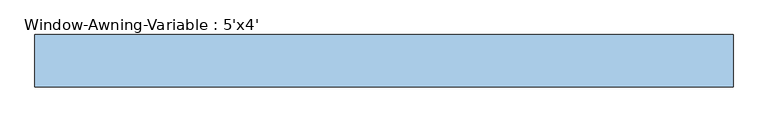
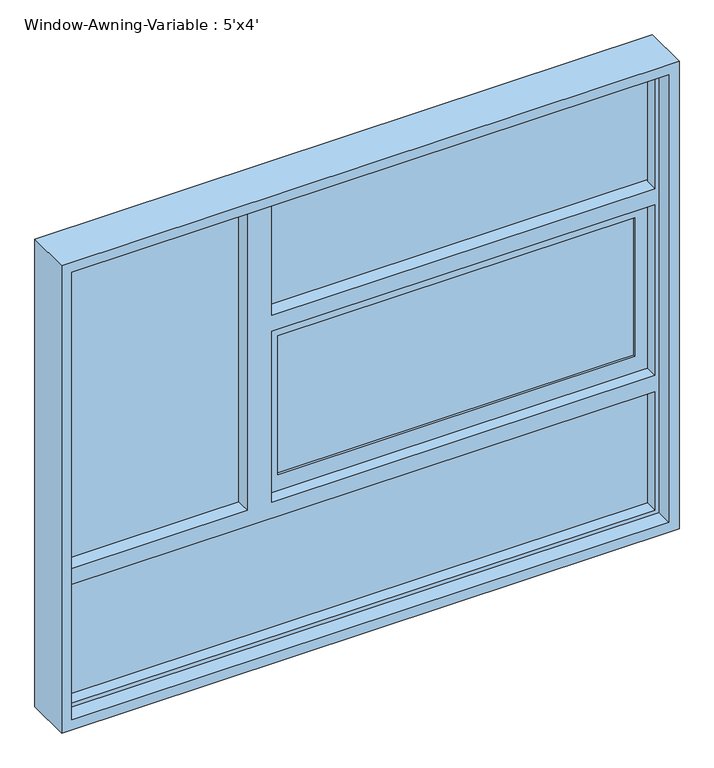
"""IFC4 building model written with IfcOpenShell, lengths in millimetres: window geometry, Window-Awning-Variable : 5'x4'."""

from ifc_helpers import new_model, si_unit, frame, origin, place, context, project, spatial, polyline, outline, extrude, faceted_brep, source, transform, mapped, element, save


def window_awning_variable_5_x4_55050b8f(model_context):
    return source(origin(), model_context, "Body", "SolidModel", [
        extrude(outline(polyline([(694.7296875, 41.275), (694.7296875, 34.925), (-186.7296875, 34.925), (-186.7296875, 41.275), (694.7296875, 41.275)])), frame((0.0, 0.0, 1342.9654688), z_axis=(0.0, 0.0, 1.0), x_axis=(1.0, 0.0, 0.0)), (0.0, 0.0, 1.0), 362.0690625),
        extrude(outline(polyline([(694.7296875, 28.575), (694.7296875, 22.225), (-186.7296875, 22.225), (-186.7296875, 28.575), (694.7296875, 28.575)])), frame((0.0, 0.0, 1342.9654688), z_axis=(0.0, 0.0, 1.0), x_axis=(1.0, 0.0, 0.0)), (0.0, 0.0, 1.0), 362.0690625),
        extrude(outline(polyline([(-279.4, 41.275), (-279.4, 34.925), (-736.6, 34.925), (-736.6, 41.275), (-279.4, 41.275)])), frame((0.0, 0.0, 1301.0951563), z_axis=(0.0, 0.0, 1.0), x_axis=(1.0, 0.0, 0.0)), (0.0, 0.0, 1.0), 807.1048438),
        extrude(outline(polyline([(-279.4, 28.575), (-279.4, 22.225), (-736.6, 22.225), (-736.6, 28.575), (-279.4, 28.575)])), frame((0.0, 0.0, 1301.0951563), z_axis=(0.0, 0.0, 1.0), x_axis=(1.0, 0.0, 0.0)), (0.0, 0.0, 1.0), 807.1048438),
        extrude(outline(polyline([(736.6, 28.575), (736.6, 22.225), (-228.6, 22.225), (-228.6, 28.575), (736.6, 28.575)])), frame((0.0, 0.0, 1788.7751563), z_axis=(0.0, 0.0, 1.0), x_axis=(1.0, 0.0, 0.0)), (0.0, 0.0, 1.0), 319.4248438),
        extrude(outline(polyline([(736.6, 41.275), (736.6, 34.925), (-228.6, 34.925), (-228.6, 41.275), (736.6, 41.275)])), frame((0.0, 0.0, 1788.7751563), z_axis=(0.0, 0.0, 1.0), x_axis=(1.0, 0.0, 0.0)), (0.0, 0.0, 1.0), 319.4248438),
        extrude(outline(polyline([(736.6, 41.275), (736.6, 34.925), (-736.6, 34.925), (-736.6, 41.275), (736.6, 41.275)])), frame((0.0, 0.0, 939.8), z_axis=(0.0, 0.0, 1.0), x_axis=(1.0, 0.0, 0.0)), (0.0, 0.0, 1.0), 319.4248438),
        extrude(outline(polyline([(736.6, 28.575), (736.6, 22.225), (-736.6, 22.225), (-736.6, 28.575), (736.6, 28.575)])), frame((0.0, 0.0, 939.8), z_axis=(0.0, 0.0, 1.0), x_axis=(1.0, 0.0, 0.0)), (0.0, 0.0, 1.0), 319.4248438),
        faceted_brep([(-736.6, 15.875, 2108.2), (-736.6, 57.15, 2108.2), (736.6, 57.15, 2108.2), (736.6, 15.875, 2108.2), (-228.6, 15.875, 2108.2), (-228.6, 53.975, 2108.2), (-279.4, 53.975, 2108.2), (-279.4, 15.875, 2108.2), (-726.4796875, -15.08125, 2098.0796875), (-726.4796875, 15.875, 2098.0796875), (-279.4, 15.875, 2098.0796875), (-279.4, -15.08125, 2098.0796875), (726.4796875, 15.875, 2098.0796875), (726.4796875, -15.08125, 2098.0796875), (-218.4796875, -15.08125, 2098.0796875), (-218.4796875, 15.875, 2098.0796875), (-736.6, -57.15, 2108.2), (-736.6, -15.08125, 2108.2), (736.6, -15.08125, 2108.2), (736.6, -57.15, 2108.2), (-762.0, 57.15, 2133.6), (-762.0, -57.15, 2133.6), (762.0, -57.15, 2133.6), (762.0, 57.15, 2133.6), (736.6, 57.15, 939.8), (736.6, 15.875, 939.8), (736.6, 15.875, 1259.2248438), (736.6, 53.975, 1259.2248438), (736.6, 53.975, 1301.0951563), (736.6, 15.875, 1301.0951563), (736.6, 15.875, 1746.9048438), (736.6, 53.975, 1746.9048438), (736.6, 53.975, 1788.7751563), (736.6, 15.875, 1788.7751563), (726.4796875, 15.875, 1788.7751563), (726.4796875, -15.08125, 1788.7751563), (726.4796875, 15.875, 949.9203125), (726.4796875, -15.08125, 949.9203125), (726.4796875, -15.08125, 1259.2248438), (726.4796875, 15.875, 1259.2248438), (726.4796875, 15.875, 1301.0951563), (726.4796875, -15.08125, 1301.0951563), (726.4796875, -15.08125, 1746.9048438), (726.4796875, 15.875, 1746.9048438), (736.6, -15.08125, 939.8), (736.6, -57.15, 939.8), (762.0, -57.15, 914.4), (762.0, 57.15, 914.4), (-736.6, 57.15, 939.8), (-736.6, 15.875, 939.8), (-726.4796875, 15.875, 949.9203125), (-726.4796875, -15.08125, 949.9203125), (-736.6, -15.08125, 939.8), (-736.6, -57.15, 939.8), (-762.0, -57.15, 914.4), (-762.0, 57.15, 914.4), (-736.6, 15.875, 1301.0951563), (-736.6, 53.975, 1301.0951563), (-736.6, 53.975, 1259.2248438), (-736.6, 15.875, 1259.2248438), (-218.4796875, 15.875, 1788.7751563), (-228.6, 15.875, 1788.7751563), (-726.4796875, 15.875, 1259.2248438), (-726.4796875, 15.875, 1301.0951563), (-218.4796875, 15.875, 1301.0951563), (-228.6, 15.875, 1301.0951563), (-228.6, 15.875, 1746.9048438), (-218.4796875, 15.875, 1746.9048438), (-726.4796875, -15.08125, 1301.0951563), (-726.4796875, -15.08125, 1259.2248438), (-218.4796875, -15.08125, 1788.7751563), (-279.4, -15.08125, 1301.0951563), (-218.4796875, -15.08125, 1301.0951563), (-218.4796875, -15.08125, 1746.9048438), (-279.4, 53.975, 1301.0951563), (-228.6, 53.975, 1788.7751563), (-228.6, 53.975, 1746.9048438), (-228.6, 53.975, 1301.0951563)], [[[0, 1, 2, 3, 4, 5, 6, 7]], [[8, 9, 10, 11]], [[12, 13, 14, 15]], [[16, 17, 18, 19]], [[20, 21, 22, 23]], [[3, 2, 24, 25, 26, 27, 28, 29, 30, 31, 32, 33]], [[13, 12, 34, 35]], [[36, 37, 38, 39]], [[40, 41, 42, 43]], [[19, 18, 44, 45]], [[23, 22, 46, 47]], [[25, 24, 48, 49]], [[37, 36, 50, 51]], [[45, 44, 52, 53]], [[47, 46, 54, 55]], [[1, 0, 56, 57, 58, 59, 49, 48]], [[12, 15, 60, 61, 4, 3, 33, 34]], [[25, 49, 59, 62, 50, 36, 39, 26]], [[56, 0, 7, 10, 9, 63]], [[29, 40, 43, 30]], [[64, 65, 66, 67]], [[9, 8, 68, 63]], [[51, 50, 62, 69]], [[52, 44, 18, 17], [14, 13, 35, 70], [37, 51, 69, 38], [68, 8, 11, 71], [72, 73, 42, 41]], [[17, 16, 53, 52]], [[22, 21, 54, 46], [16, 19, 45, 53]], [[21, 20, 55, 54]], [[20, 23, 47, 55], [2, 1, 48, 24]], [[58, 27, 26, 39, 38, 69, 62, 59]], [[27, 58, 57, 74, 6, 5, 75, 32, 31, 76, 77, 28]], [[29, 28, 77, 65, 64, 72, 41, 40]], [[57, 56, 63, 68, 71, 74]], [[6, 74, 71, 11, 10, 7]], [[15, 14, 70, 60]], [[72, 64, 67, 73]], [[5, 4, 61, 75]], [[65, 77, 76, 66]], [[76, 31, 30, 43, 42, 73, 67, 66]], [[32, 75, 61, 60, 70, 35, 34, 33]]]),
        extrude(outline(polyline([(1301.0951563, -228.6), (1301.0951563, 736.6), (1746.9048438, 736.6), (1746.9048438, -228.6), (1301.0951563, -228.6)]), holes=[polyline([(1342.9654688, -186.7296875), (1705.0345313, -186.7296875), (1705.0345313, 694.7296875), (1342.9654688, 694.7296875), (1342.9654688, -186.7296875)])]), frame((0.0, 15.875, 0.0), z_axis=(0.0, 1.0, 0.0), x_axis=(0.0, 0.0, 1.0)), (0.0, 0.0, 1.0), 31.75),
    ])


if __name__ == "__main__":
    model = new_model("IFC4")
    model_context = context("Model", 3, world=origin())
    ifc_project = project(units=[si_unit("LENGTHUNIT", "METRE", prefix="MILLI")], contexts=[model_context])
    site = spatial("IfcSite", under=ifc_project)
    building = spatial("IfcBuilding", under=site)
    placement = place(None, origin())
    window_awning_variable_5_x4_shape = window_awning_variable_5_x4_55050b8f(model_context)
    element("IfcWindow", 1, ObjectType="Window-Awning-Variable : 5'x4'", at=placement, inside=building, context=model_context, shape_type="MappedRepresentation", body=[
        mapped(window_awning_variable_5_x4_shape, transform((0.0, 0.0, 0.0), x_axis=(1.0, 0.0, 0.0), y_axis=(0.0, 1.0, 0.0), z_axis=(0.0, 0.0, 1.0))),
    ])
    save(model, "model.ifc")

# Revit data of these elements
# Type "Window-Awning-Variable : 5'x4'"
#   Type Mark = "23"
#   Fire Rating = "0.5h"
#   Assembly Code = "B2020100"
#   Analytic Construction = "Double glazing - domestic"
#   Window Inset [instance default] = 0' - 0 5/8"
#   Wall Thickness [instance default] = 0' - 6"
#   Visual Light Transmittance = 0.81
#   Transom Height Ratio = 0.3
#   Transom Height = 1' - 2.4"
#   Thermal Resistance (R) = 1.8146 (h·ft²·°F)/BTU
#   Solar Heat Gain Coefficient = 0.76
#   Rough Width = 5' - 0 1/2"
#   Rough Height = 4' - 0 1/2"
#   Opening Window Width = 3' - 4"
#   Opening Window Height = 1' - 7.2"
#   Heat Transfer Coefficient (U) = 0.5511 BTU/(h·ft²·°F)
#   Height = 4' - 0"
#   Frame Gap 3 [instance default] = 0' - 1 83/128"
#   Frame Gap 2 [instance default] = 0' - 0 5/8"
#   Frame Gap 1 = 0' - 1 51/128"
#   Fixed Window Width = 1' - 8"
#   Default Sill Height = 3' - 0"
#   Width = 5' - 0"
#   Frame Material = Metal - Aluminum
#   Glass Panel Material = Glass
#   Wall Closure = (empty or 0)
# Element 1 (IfcWindow, "Window-Awning-Variable : 5'x4'")
#   Wall Thickness = 0' - 4 1/2"
#   Materials on its faces: "Glass", "Metal - Aluminum"
# Materials
#   "Metal - Aluminum": class "Metal", colour RGB 247 247 247, transparency 0
#   "Glass": class "Glass", colour RGB 0 128 192, transparency 0.75, Description = "Soda Lime Glass", Cost = 0
